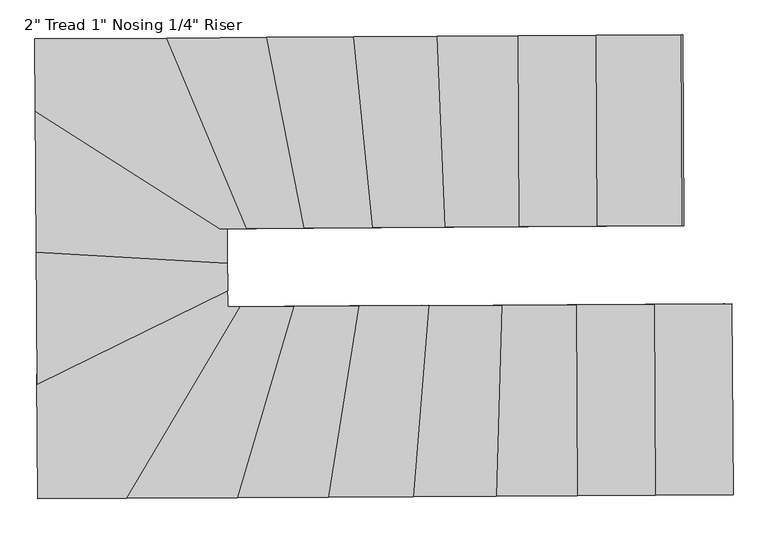
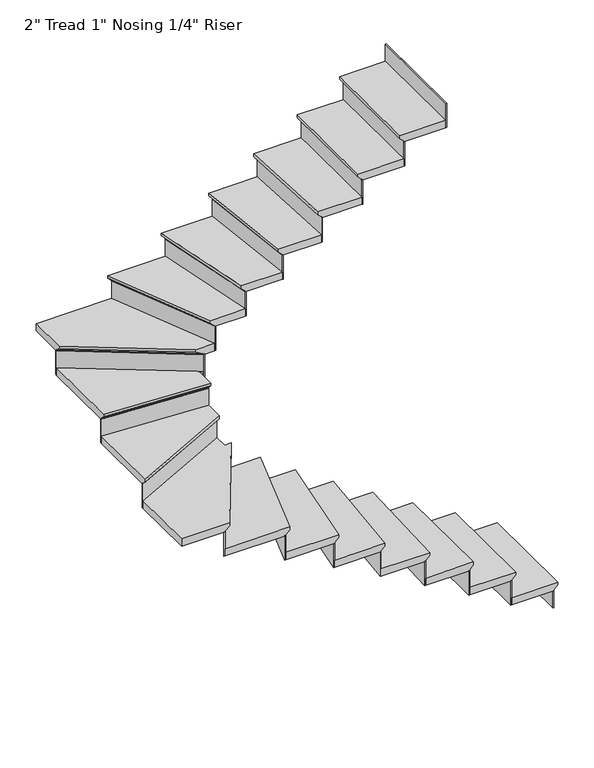
"""IFC4 building model written with IfcOpenShell, lengths in millimetres: stair flight geometry."""

from ifc_helpers import new_model, si_unit, origin, place, context, project, spatial, faceted_brep, source, transform, mapped, element, save


def stair_flight_a1ba2c50(model_context):
    return source(origin(), model_context, "Body", "Brep", [
        faceted_brep([(-120.6930289, -3539.621908, 6551.0833333), (-120.6930289, -3539.621908, 6570.1333333), (-116.4891496, -4225.4090232, 6570.1333333), (-116.4891496, -4225.4090232, 6551.0833333), (-146.0925517, -3539.7776072, 6525.6833333), (-141.8886723, -4225.5647224, 6525.6833333), (-425.4873024, -3541.4902988, 6570.1333333), (-421.283423, -4227.277414, 6570.1333333), (-141.8886723, -4225.5647224, 6519.3333333), (-421.283423, -4227.277414, 6519.3333333), (-425.4873024, -3541.4902988, 6519.3333333), (-146.0925517, -3539.7776072, 6519.3333333)], [[[0, 1, 2, 3]], [[4, 0, 3, 5]], [[2, 1, 6, 7]], [[8, 9, 10, 11]], [[2, 7, 9, 8, 5, 3]], [[8, 11, 4, 5]], [[6, 1, 0, 4, 11, 10]], [[7, 6, 10, 9]]]),
        faceted_brep([(-146.0925517, -3539.7776072, 6519.3333333), (-146.0925517, -3539.7776072, 6400.8), (-152.4424324, -3539.816532, 6400.8), (-152.4424324, -3539.816532, 6519.3333333), (-141.8886723, -4225.5647224, 6519.3333333), (-148.238553, -4225.6036472, 6519.3333333), (-148.238553, -4225.6036472, 6400.8), (-141.8886723, -4225.5647224, 6400.8)], [[[0, 1, 2, 3]], [[4, 5, 6, 7]], [[1, 0, 4, 7]], [[2, 1, 7, 6]], [[3, 2, 6, 5]], [[0, 3, 5, 4]]]),
        faceted_brep([(-425.4873024, -3541.4902988, 6688.6666667), (-425.4873024, -3541.4902988, 6519.3333333), (-431.8371831, -3541.5292236, 6519.3333333), (-431.8371831, -3541.5292236, 6688.6666667), (-421.283423, -4227.277414, 6688.6666667), (-427.6333037, -4227.3163388, 6688.6666667), (-427.6333037, -4227.3163388, 6519.3333333), (-421.283423, -4227.277414, 6519.3333333)], [[[0, 1, 2, 3]], [[4, 5, 6, 7]], [[1, 0, 4, 7]], [[2, 1, 7, 6]], [[3, 2, 6, 5]], [[0, 3, 5, 4]]]),
        faceted_brep([(-395.8839002, -4227.1217148, 6739.4666667), (-400.0877796, -3541.3345996, 6739.4666667), (-704.882053, -3543.2029904, 6739.4666667), (-700.6781736, -4228.9901056, 6739.4666667), (-421.283423, -4227.277414, 6688.6666667), (-700.6781736, -4228.9901056, 6688.6666667), (-704.882053, -3543.2029904, 6688.6666667), (-425.4873024, -3541.4902988, 6688.6666667), (-421.283423, -4227.277414, 6695.0166667), (-395.8839002, -4227.1217148, 6720.4166667), (-425.4873024, -3541.4902988, 6695.0166667), (-400.0877796, -3541.3345996, 6720.4166667)], [[[0, 1, 2, 3]], [[4, 5, 6, 7]], [[0, 3, 5, 4, 8, 9]], [[4, 7, 10, 8]], [[2, 1, 11, 10, 7, 6]], [[3, 2, 6, 5]], [[11, 1, 0, 9]], [[10, 11, 9, 8]]]),
        faceted_brep([(-704.882053, -3543.2029904, 6858.0), (-704.882053, -3543.2029904, 6688.6666667), (-711.2319337, -3543.2419152, 6688.6666667), (-711.2319337, -3543.2419152, 6858.0), (-700.6781736, -4228.9901056, 6858.0), (-707.0280543, -4229.0290304, 6858.0), (-707.0280543, -4229.0290304, 6688.6666667), (-700.6781736, -4228.9901056, 6688.6666667)], [[[0, 1, 2, 3]], [[4, 5, 6, 7]], [[1, 0, 4, 7]], [[2, 1, 7, 6]], [[3, 2, 6, 5]], [[0, 3, 5, 4]]]),
        faceted_brep([(-675.2786508, -4228.8344064, 6908.8), (-679.4825302, -3543.0472912, 6908.8), (-971.9344004, -3544.840023, 6908.8), (-992.4483132, -4230.7786584, 6908.8), (-700.6781736, -4228.9901056, 6858.0), (-992.4483132, -4230.7786584, 6858.0), (-971.9344004, -3544.840023, 6858.0), (-704.882053, -3543.2029904, 6858.0), (-700.6781736, -4228.9901056, 6864.35), (-675.2786508, -4228.8344064, 6889.75), (-704.882053, -3543.2029904, 6864.35), (-679.4825302, -3543.0472912, 6889.75)], [[[0, 1, 2, 3]], [[4, 5, 6, 7]], [[0, 3, 5, 4, 8, 9]], [[4, 7, 10, 8]], [[2, 1, 11, 10, 7, 6]], [[3, 2, 6, 5]], [[11, 1, 0, 9]], [[10, 11, 9, 8]]]),
        faceted_brep([(-971.9344004, -3544.840023, 7027.3333333), (-971.9344004, -3544.840023, 6858.0), (-978.2884043, -3544.8789731, 6858.0), (-978.2884043, -3544.8789731, 7027.3333333), (-992.4483132, -4230.7786584, 7027.3333333), (-998.8023171, -4230.8176085, 7027.3333333), (-998.8023171, -4230.8176085, 6858.0), (-992.4483132, -4230.7786584, 6858.0)], [[[0, 1, 2, 3]], [[4, 5, 6, 7]], [[1, 0, 4, 7]], [[2, 1, 7, 6]], [[3, 2, 6, 5]], [[0, 3, 5, 4]]]),
        faceted_brep([(-967.0322975, -4230.6228581, 7078.1333333), (-946.5183848, -3544.6842227, 7078.1333333), (-1233.842238, -3546.4455197, 7078.1333333), (-1289.4900883, -4232.5995264, 7078.1333333), (-992.4483132, -4230.7786584, 7027.3333333), (-1289.4900883, -4232.5995264, 7027.3333333), (-1233.842238, -3546.4455197, 7027.3333333), (-971.9344004, -3544.840023, 7027.3333333), (-992.4483132, -4230.7786584, 7033.6833333), (-967.0322975, -4230.6228581, 7059.0833333), (-971.9344004, -3544.840023, 7033.6833333), (-946.5183848, -3544.6842227, 7059.0833333)], [[[0, 1, 2, 3]], [[4, 5, 6, 7]], [[0, 3, 5, 4, 8, 9]], [[4, 7, 10, 8]], [[2, 1, 11, 10, 7, 6]], [[3, 2, 6, 5]], [[11, 1, 0, 9]], [[10, 11, 9, 8]]]),
        faceted_brep([(-1233.842238, -3546.4455197, 7196.6666667), (-1233.842238, -3546.4455197, 7027.3333333), (-1240.2162558, -3546.4845925, 7027.3333333), (-1240.2162558, -3546.4845925, 7196.6666667), (-1289.4900883, -4232.5995264, 7196.6666667), (-1295.8641061, -4232.6385992, 7196.6666667), (-1295.8641061, -4232.6385992, 7027.3333333), (-1289.4900883, -4232.5995264, 7027.3333333)], [[[0, 1, 2, 3]], [[4, 5, 6, 7]], [[1, 0, 4, 7]], [[2, 1, 7, 6]], [[3, 2, 6, 5]], [[0, 3, 5, 4]]]),
        faceted_brep([(-1263.994017, -4232.4432353, 7247.4666667), (-1208.3461666, -3546.2892286, 7247.4666667), (-1486.5415383, -3547.994568, 7247.4666667), (-1596.081167, -4234.4789317, 7247.4666667), (-1289.4900883, -4232.5995264, 7196.6666667), (-1596.081167, -4234.4789317, 7196.6666667), (-1486.5415383, -3547.994568, 7196.6666667), (-1233.842238, -3546.4455197, 7196.6666667), (-1289.4900883, -4232.5995264, 7203.0166667), (-1263.994017, -4232.4432353, 7228.4166667), (-1233.842238, -3546.4455197, 7203.0166667), (-1208.3461666, -3546.2892286, 7228.4166667)], [[[0, 1, 2, 3]], [[4, 5, 6, 7]], [[0, 3, 5, 4, 8, 9]], [[4, 7, 10, 8]], [[2, 1, 11, 10, 7, 6]], [[3, 2, 6, 5]], [[11, 1, 0, 9]], [[10, 11, 9, 8]]]),
        faceted_brep([(-1486.5415383, -3547.994568, 7366.0), (-1486.5415383, -3547.994568, 7196.6666667), (-1492.9781659, -3548.0340246, 7196.6666667), (-1492.9781659, -3548.0340246, 7366.0), (-1596.081167, -4234.4789317, 7366.0), (-1602.5177946, -4234.5183882, 7366.0), (-1602.5177946, -4234.5183882, 7196.6666667), (-1596.081167, -4234.4789317, 7196.6666667)], [[[0, 1, 2, 3]], [[4, 5, 6, 7]], [[1, 0, 4, 7]], [[2, 1, 7, 6]], [[3, 2, 6, 5]], [[0, 3, 5, 4]]]),
        faceted_brep([(-1570.3346568, -4234.3211054, 7416.8), (-1460.7950281, -3547.8367418, 7416.8), (-1720.1488607, -3549.4265824, 7416.8), (-1922.8306159, -4236.4819079, 7416.8), (-1596.081167, -4234.4789317, 7366.0), (-1922.8306159, -4236.4819079, 7366.0), (-1720.1488607, -3549.4265824, 7366.0), (-1486.5415383, -3547.994568, 7366.0), (-1596.081167, -4234.4789317, 7372.35), (-1570.3346568, -4234.3211054, 7397.75), (-1486.5415383, -3547.994568, 7372.35), (-1460.7950281, -3547.8367418, 7397.75)], [[[0, 1, 2, 3]], [[4, 5, 6, 7]], [[0, 3, 5, 4, 8, 9]], [[4, 7, 10, 8]], [[2, 1, 11, 10, 7, 6]], [[3, 2, 6, 5]], [[11, 1, 0, 9]], [[10, 11, 9, 8]]]),
        faceted_brep([(-1720.1488607, -3549.4265824, 7535.3333333), (-1720.1488607, -3549.4265824, 7366.0), (-1726.781397, -3549.4672399, 7366.0), (-1726.781397, -3549.4672399, 7535.3333333), (-1922.8306159, -4236.4819079, 7535.3333333), (-1929.4631522, -4236.5225654, 7535.3333333), (-1929.4631522, -4236.5225654, 7366.0), (-1922.8306159, -4236.4819079, 7366.0)], [[[0, 1, 2, 3]], [[4, 5, 6, 7]], [[1, 0, 4, 7]], [[2, 1, 7, 6]], [[3, 2, 6, 5]], [[0, 3, 5, 4]]]),
        faceted_brep([(-1896.3004707, -4236.3192779, 7586.1333333), (-1693.6187155, -3549.2639524, 7586.1333333), (-1917.3665941, -3550.6355283, 7586.1333333), (-2324.8688668, -4238.9464049, 7586.1333333), (-1922.8306159, -4236.4819079, 7535.3333333), (-2324.8688668, -4238.9464049, 7535.3333333), (-1917.3665941, -3550.6355283, 7535.3333333), (-1720.1488607, -3549.4265824, 7535.3333333), (-1922.8306159, -4236.4819079, 7541.6833333), (-1896.3004707, -4236.3192779, 7567.0833333), (-1720.1488607, -3549.4265824, 7541.6833333), (-1693.6187155, -3549.2639524, 7567.0833333)], [[[0, 1, 2, 3]], [[4, 5, 6, 7]], [[0, 3, 5, 4, 8, 9]], [[4, 7, 10, 8]], [[2, 1, 11, 10, 7, 6]], [[3, 2, 6, 5]], [[11, 1, 0, 9]], [[10, 11, 9, 8]]]),
        faceted_brep([(-1917.3665941, -3550.6355283, 7704.6666667), (-1917.3665941, -3550.6355283, 7535.3333333), (-1924.7728783, -3550.6809289, 7535.3333333), (-1924.7728783, -3550.6809289, 7704.6666667), (-2324.8688668, -4238.9464049, 7704.6666667), (-2332.275151, -4238.9918055, 7704.6666667), (-2332.275151, -4238.9918055, 7535.3333333), (-2324.8688668, -4238.9464049, 7535.3333333)], [[[0, 1, 2, 3]], [[4, 5, 6, 7]], [[1, 0, 4, 7]], [[2, 1, 7, 6]], [[3, 2, 6, 5]], [[0, 3, 5, 4]]]),
        faceted_brep([(-2615.3480869, -3801.2875551, 7755.4666667), (-2612.6544213, -4240.7105322, 7755.4666667), (-2295.24373, -4238.7648026, 7755.4666667), (-1887.7414574, -3550.4539261, 7755.4666667), (-1931.0711854, -3550.7195376, 7755.4666667), (-1931.5966592, -3464.9979706, 7755.4666667), (-2612.6544213, -4240.7105322, 7704.6666667), (-2615.3480869, -3801.2875551, 7704.6666667), (-1931.5966592, -3464.9979706, 7704.6666667), (-1931.0711854, -3550.7195376, 7704.6666667), (-1917.3665941, -3550.6355283, 7704.6666667), (-2324.8688668, -4238.9464049, 7704.6666667), (-1917.3665941, -3550.6355283, 7711.0166667), (-2324.8688668, -4238.9464049, 7711.0166667), (-1887.7414574, -3550.4539261, 7736.4166667), (-2295.24373, -4238.7648026, 7736.4166667)], [[[0, 1, 2, 3, 4, 5]], [[6, 7, 8, 9, 10, 11]], [[1, 0, 7, 6]], [[11, 10, 12, 13]], [[5, 4, 9, 8]], [[0, 5, 8, 7]], [[14, 3, 2, 15]], [[12, 14, 15, 13]], [[4, 3, 14, 12, 10, 9]], [[2, 1, 6, 11, 13, 15]]]),
        faceted_brep([(-1931.5966592, -3464.9979706, 7874.0), (-1931.5966592, -3464.9979706, 7704.6666667), (-1931.6399076, -3457.9427742, 7704.6666667), (-1931.6399076, -3457.9427742, 7874.0), (-2615.3480869, -3801.2875551, 7874.0), (-2615.3913353, -3794.2323587, 7874.0), (-2615.3913353, -3794.2323587, 7704.6666667), (-2615.3480869, -3801.2875551, 7704.6666667)], [[[0, 1, 2, 3]], [[4, 5, 6, 7]], [[1, 0, 4, 7]], [[2, 1, 7, 6]], [[3, 2, 6, 5]], [[0, 3, 5, 4]]]),
        faceted_brep([(-2615.1750933, -3829.5083406, 7924.8), (-1931.4236656, -3493.2187561, 7924.8), (-1932.1828972, -3369.3638122, 7924.8), (-2618.2387587, -3329.7265819, 7924.8), (-2615.3480869, -3801.2875551, 7874.0), (-2618.2387587, -3329.7265819, 7874.0), (-1932.1828972, -3369.3638122, 7874.0), (-1931.5966592, -3464.9979706, 7874.0), (-2615.3480869, -3801.2875551, 7880.35), (-2615.1750933, -3829.5083406, 7905.75), (-1931.5966592, -3464.9979706, 7880.35), (-1931.4236656, -3493.2187561, 7905.75)], [[[0, 1, 2, 3]], [[4, 5, 6, 7]], [[0, 3, 5, 4, 8, 9]], [[4, 7, 10, 8]], [[2, 1, 11, 10, 7, 6]], [[3, 2, 6, 5]], [[11, 1, 0, 9]], [[10, 11, 9, 8]]]),
        faceted_brep([(-1932.1828972, -3369.3638122, 8043.3333333), (-1932.1828972, -3369.3638122, 7874.0), (-1932.2219015, -3363.0009693, 7874.0), (-1932.2219015, -3363.0009693, 8043.3333333), (-2618.2387587, -3329.7265819, 8043.3333333), (-2618.277763, -3323.363739, 8043.3333333), (-2618.277763, -3323.363739, 7874.0), (-2618.2387587, -3329.7265819, 7874.0)], [[[0, 1, 2, 3]], [[4, 5, 6, 7]], [[1, 0, 4, 7]], [[2, 1, 7, 6]], [[3, 2, 6, 5]], [[0, 3, 5, 4]]]),
        faceted_brep([(-2618.0827416, -3355.1779533, 8094.1333333), (-1932.0268801, -3394.8151835, 8094.1333333), (-1932.783877, -3271.3247869, 8094.1333333), (-1912.0496222, -3271.1976858, 8094.1333333), (-2621.364296, -2819.8515342, 8094.1333333), (-2618.2387587, -3329.7265819, 8043.3333333), (-2621.364296, -2819.8515342, 8043.3333333), (-1912.0496222, -3271.1976858, 8043.3333333), (-1932.783877, -3271.3247869, 8043.3333333), (-1932.1828972, -3369.3638122, 8043.3333333), (-2618.2387587, -3329.7265819, 8049.6833333), (-2618.0827416, -3355.1779533, 8075.0833333), (-1932.1828972, -3369.3638122, 8049.6833333), (-1932.0268801, -3394.8151835, 8075.0833333)], [[[0, 1, 2, 3, 4]], [[5, 6, 7, 8, 9]], [[0, 4, 6, 5, 10, 11]], [[5, 9, 12, 10]], [[2, 1, 13, 12, 9, 8]], [[3, 2, 8, 7]], [[4, 3, 7, 6]], [[13, 1, 0, 11]], [[12, 13, 11, 10]]]),
        faceted_brep([(-1912.0496222, -3271.1976858, 8212.6666667), (-1912.0496222, -3271.1976858, 8043.3333333), (-1900.3341194, -3271.1258697, 8043.3333333), (-1900.3341194, -3271.1258697, 8212.6666667), (-2621.364296, -2819.8515342, 8212.6666667), (-2621.4106144, -2812.2955182, 8212.6666667), (-2621.4106144, -2812.2955182, 8043.3333333), (-2621.364296, -2819.8515342, 8043.3333333)], [[[0, 1, 2, 3]], [[4, 5, 6, 7]], [[1, 0, 4, 7]], [[2, 1, 7, 6]], [[3, 2, 6, 5]], [[0, 3, 5, 4]]]),
        faceted_brep([(-2121.4312205, -2586.6683113, 8263.4666667), (-2622.7748716, -2589.7415511, 8263.4666667), (-2621.1790223, -2850.0755978, 8263.4666667), (-1958.9116334, -3271.4849502, 8263.4666667), (-1835.3232791, -3270.7273529, 8263.4666667), (-2622.7748716, -2589.7415511, 8212.6666667), (-2121.4312205, -2586.6683113, 8212.6666667), (-1835.3232791, -3270.7273529, 8212.6666667), (-1912.0496222, -3271.1976858, 8212.6666667), (-2621.364296, -2819.8515342, 8212.6666667), (-2621.364296, -2819.8515342, 8219.0166667), (-2621.1790223, -2850.0755978, 8244.4166667), (-1912.0496222, -3271.1976858, 8219.0166667), (-1958.9116334, -3271.4849502, 8244.4166667)], [[[0, 1, 2, 3, 4]], [[5, 6, 7, 8, 9]], [[1, 0, 6, 5]], [[2, 1, 5, 9, 10, 11]], [[9, 8, 12, 10]], [[0, 4, 7, 6]], [[13, 3, 2, 11]], [[12, 13, 11, 10]], [[4, 3, 13, 12, 8, 7]]]),
        faceted_brep([(-1835.3232791, -3270.7273529, 8382.0), (-1835.3232791, -3270.7273529, 8212.6666667), (-1828.4578405, -3270.6852677, 8212.6666667), (-1828.4578405, -3270.6852677, 8382.0), (-2121.4312205, -2586.6683113, 8382.0), (-2114.5657819, -2586.6262261, 8382.0), (-2114.5657819, -2586.6262261, 8212.6666667), (-2121.4312205, -2586.6683113, 8212.6666667)], [[[0, 1, 2, 3]], [[4, 5, 6, 7]], [[1, 0, 4, 7]], [[2, 1, 7, 6]], [[3, 2, 6, 5]], [[0, 3, 5, 4]]]),
        faceted_brep([(-2148.8929752, -2586.8366521, 8432.8), (-1862.7850338, -3270.8956936, 8432.8), (-1630.6514822, -3269.4727134, 8432.8), (-1765.0751589, -2584.4838464, 8432.8), (-2121.4312205, -2586.6683113, 8382.0), (-1765.0751589, -2584.4838464, 8382.0), (-1630.6514822, -3269.4727134, 8382.0), (-1835.3232791, -3270.7273529, 8382.0), (-2121.4312205, -2586.6683113, 8388.35), (-2148.8929752, -2586.8366521, 8413.75), (-1835.3232791, -3270.7273529, 8388.35), (-1862.7850338, -3270.8956936, 8413.75)], [[[0, 1, 2, 3]], [[4, 5, 6, 7]], [[0, 3, 5, 4, 8, 9]], [[4, 7, 10, 8]], [[2, 1, 11, 10, 7, 6]], [[3, 2, 6, 5]], [[11, 1, 0, 9]], [[10, 11, 9, 8]]]),
        faceted_brep([(-1630.6514822, -3269.4727134, 8551.3333333), (-1630.6514822, -3269.4727134, 8382.0), (-1624.1881401, -3269.4330931, 8382.0), (-1624.1881401, -3269.4330931, 8551.3333333), (-1765.0751589, -2584.4838464, 8551.3333333), (-1758.6118168, -2584.4442261, 8551.3333333), (-1758.6118168, -2584.4442261, 8382.0), (-1765.0751589, -2584.4838464, 8382.0)], [[[0, 1, 2, 3]], [[4, 5, 6, 7]], [[1, 0, 4, 7]], [[2, 1, 7, 6]], [[3, 2, 6, 5]], [[0, 3, 5, 4]]]),
        faceted_brep([(-1790.9285273, -2584.6423277, 8602.1333333), (-1656.5048506, -3269.6311948, 8602.1333333), (-1385.319119, -3267.9688245, 8602.1333333), (-1452.3132293, -2582.5666138, 8602.1333333), (-1765.0751589, -2584.4838464, 8551.3333333), (-1452.3132293, -2582.5666138, 8551.3333333), (-1385.319119, -3267.9688245, 8551.3333333), (-1630.6514822, -3269.4727134, 8551.3333333), (-1765.0751589, -2584.4838464, 8557.6833333), (-1790.9285273, -2584.6423277, 8583.0833333), (-1630.6514822, -3269.4727134, 8557.6833333), (-1656.5048506, -3269.6311948, 8583.0833333)], [[[0, 1, 2, 3]], [[4, 5, 6, 7]], [[0, 3, 5, 4, 8, 9]], [[4, 7, 10, 8]], [[2, 1, 11, 10, 7, 6]], [[3, 2, 6, 5]], [[11, 1, 0, 9]], [[10, 11, 9, 8]]]),
        faceted_brep([(-1385.319119, -3267.9688245, 8720.6666667), (-1385.319119, -3267.9688245, 8551.3333333), (-1378.942678, -3267.9297369, 8551.3333333), (-1378.942678, -3267.9297369, 8720.6666667), (-1452.3132293, -2582.5666138, 8720.6666667), (-1445.9367882, -2582.5275262, 8720.6666667), (-1445.9367882, -2582.5275262, 8551.3333333), (-1452.3132293, -2582.5666138, 8551.3333333)], [[[0, 1, 2, 3]], [[4, 5, 6, 7]], [[1, 0, 4, 7]], [[2, 1, 7, 6]], [[3, 2, 6, 5]], [[0, 3, 5, 4]]]),
        faceted_brep([(-1477.8189934, -2582.7229643, 8771.4666667), (-1410.8248832, -3268.125175, 8771.4666667), (-1125.1141805, -3266.3737666, 8771.4666667), (-1153.9085026, -2580.7373909, 8771.4666667), (-1452.3132293, -2582.5666138, 8720.6666667), (-1153.9085026, -2580.7373909, 8720.6666667), (-1125.1141805, -3266.3737666, 8720.6666667), (-1385.319119, -3267.9688245, 8720.6666667), (-1452.3132293, -2582.5666138, 8727.0166667), (-1477.8189934, -2582.7229643, 8752.4166667), (-1385.319119, -3267.9688245, 8727.0166667), (-1410.8248832, -3268.125175, 8752.4166667)], [[[0, 1, 2, 3]], [[4, 5, 6, 7]], [[0, 3, 5, 4, 8, 9]], [[4, 7, 10, 8]], [[2, 1, 11, 10, 7, 6]], [[3, 2, 6, 5]], [[11, 1, 0, 9]], [[10, 11, 9, 8]]]),
        faceted_brep([(-1125.1141805, -3266.3737666, 8890.0), (-1125.1141805, -3266.3737666, 8720.6666667), (-1118.7602189, -3266.3348167, 8720.6666667), (-1118.7602189, -3266.3348167, 8890.0), (-1153.9085026, -2580.7373909, 8890.0), (-1147.554541, -2580.6984411, 8890.0), (-1147.554541, -2580.6984411, 8720.6666667), (-1153.9085026, -2580.7373909, 8720.6666667)], [[[0, 1, 2, 3]], [[4, 5, 6, 7]], [[1, 0, 4, 7]], [[2, 1, 7, 6]], [[3, 2, 6, 5]], [[0, 3, 5, 4]]]),
        faceted_brep([(-1179.3243487, -2580.8931902, 8940.8), (-1150.5300267, -3266.5295659, 8940.8), (-858.0309746, -3264.7365448, 8940.8), (-862.2348539, -2578.9494296, 8940.8), (-1153.9085026, -2580.7373909, 8890.0), (-862.2348539, -2578.9494296, 8890.0), (-858.0309746, -3264.7365448, 8890.0), (-1125.1141805, -3266.3737666, 8890.0), (-1153.9085026, -2580.7373909, 8896.35), (-1179.3243487, -2580.8931902, 8921.75), (-1125.1141805, -3266.3737666, 8896.35), (-1150.5300267, -3266.5295659, 8921.75)], [[[0, 1, 2, 3]], [[4, 5, 6, 7]], [[0, 3, 5, 4, 8, 9]], [[4, 7, 10, 8]], [[2, 1, 11, 10, 7, 6]], [[3, 2, 6, 5]], [[11, 1, 0, 9]], [[10, 11, 9, 8]]]),
        faceted_brep([(-858.0309746, -3264.7365448, 9059.3333333), (-858.0309746, -3264.7365448, 8890.0), (-851.6810939, -3264.69762, 8890.0), (-851.6810939, -3264.69762, 9059.3333333), (-862.2348539, -2578.9494296, 9059.3333333), (-855.8849733, -2578.9105048, 9059.3333333), (-855.8849733, -2578.9105048, 8890.0), (-862.2348539, -2578.9494296, 8890.0)], [[[0, 1, 2, 3]], [[4, 5, 6, 7]], [[1, 0, 4, 7]], [[2, 1, 7, 6]], [[3, 2, 6, 5]], [[0, 3, 5, 4]]]),
        faceted_brep([(-887.6343767, -2579.1051288, 9110.1333333), (-883.4304974, -3264.8922441, 9110.1333333), (-578.6362239, -3263.0238532, 9110.1333333), (-582.8401033, -2577.236738, 9110.1333333), (-862.2348539, -2578.9494296, 9059.3333333), (-582.8401033, -2577.236738, 9059.3333333), (-578.6362239, -3263.0238532, 9059.3333333), (-858.0309746, -3264.7365448, 9059.3333333), (-862.2348539, -2578.9494296, 9065.6833333), (-887.6343767, -2579.1051288, 9091.0833333), (-858.0309746, -3264.7365448, 9065.6833333), (-883.4304974, -3264.8922441, 9091.0833333)], [[[0, 1, 2, 3]], [[4, 5, 6, 7]], [[0, 3, 5, 4, 8, 9]], [[4, 7, 10, 8]], [[2, 1, 11, 10, 7, 6]], [[3, 2, 6, 5]], [[11, 1, 0, 9]], [[10, 11, 9, 8]]]),
        faceted_brep([(-578.6362239, -3263.0238532, 9228.6666667), (-578.6362239, -3263.0238532, 9059.3333333), (-572.2863432, -3262.9849284, 9059.3333333), (-572.2863432, -3262.9849284, 9228.6666667), (-582.8401033, -2577.236738, 9228.6666667), (-576.4902226, -2577.1978132, 9228.6666667), (-576.4902226, -2577.1978132, 9059.3333333), (-582.8401033, -2577.236738, 9059.3333333)], [[[0, 1, 2, 3]], [[4, 5, 6, 7]], [[1, 0, 4, 7]], [[2, 1, 7, 6]], [[3, 2, 6, 5]], [[0, 3, 5, 4]]]),
        faceted_brep([(-299.2414733, -3261.3111616, 9398.0), (-299.2414733, -3261.3111616, 9228.6666667), (-292.8915926, -3261.2722368, 9228.6666667), (-292.8915926, -3261.2722368, 9398.0), (-303.4453527, -2575.5240464, 9398.0), (-297.095472, -2575.4851216, 9398.0), (-297.095472, -2575.4851216, 9228.6666667), (-303.4453527, -2575.5240464, 9228.6666667)], [[[0, 1, 2, 3]], [[4, 5, 6, 7]], [[1, 0, 4, 7]], [[2, 1, 7, 6]], [[3, 2, 6, 5]], [[0, 3, 5, 4]]]),
        faceted_brep([(-608.2396261, -2577.3924372, 9279.4666667), (-604.0357467, -3263.1795525, 9279.4666667), (-299.2414733, -3261.3111616, 9279.4666667), (-303.4453527, -2575.5240464, 9279.4666667), (-582.8401033, -2577.236738, 9228.6666667), (-303.4453527, -2575.5240464, 9228.6666667), (-299.2414733, -3261.3111616, 9228.6666667), (-578.6362239, -3263.0238532, 9228.6666667), (-582.8401033, -2577.236738, 9235.0166667), (-608.2396261, -2577.3924372, 9260.4166667), (-578.6362239, -3263.0238532, 9235.0166667), (-604.0357467, -3263.1795525, 9260.4166667)], [[[0, 1, 2, 3]], [[4, 5, 6, 7]], [[0, 3, 5, 4, 8, 9]], [[4, 7, 10, 8]], [[2, 1, 11, 10, 7, 6]], [[3, 2, 6, 5]], [[11, 1, 0, 9]], [[10, 11, 9, 8]]]),
    ])


if __name__ == "__main__":
    model = new_model("IFC4")
    model_context = context("Model", 3, world=origin())
    ifc_project = project(units=[si_unit("LENGTHUNIT", "METRE", prefix="MILLI")], contexts=[model_context])
    site = spatial("IfcSite", under=ifc_project)
    building = spatial("IfcBuilding", under=site)
    placement = place(None, origin())
    stair_flight_shape = stair_flight_a1ba2c50(model_context)
    element("IfcStairFlight", 1, ObjectType="2\" Tread 1\" Nosing 1/4\" Riser", at=placement, inside=building, context=model_context, shape_type="MappedRepresentation", body=[
        mapped(stair_flight_shape, transform((0.0, 0.0, 0.0), x_axis=(1.0, 0.0, 0.0), y_axis=(0.0, 1.0, 0.0), z_axis=(0.0, 0.0, 1.0))),
    ])
    save(model, "model.ifc")
